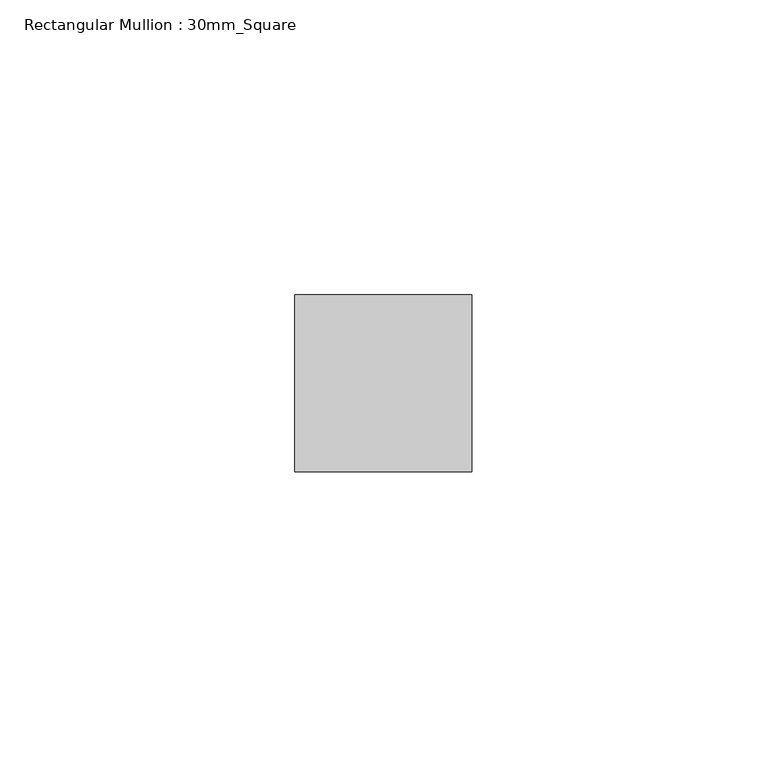
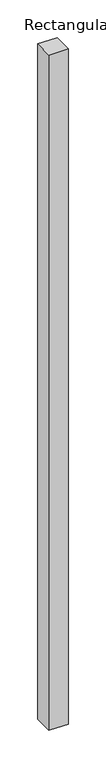
"""IFC4 building model written with IfcOpenShell, lengths in millimetres: member geometry, Rectangular Mullion : 30mm_Square."""

from ifc_helpers import new_model, si_unit, frame, origin, place, context, project, spatial, polyline, outline, extrude, source, transform, mapped, element, save


def rectangular_mullion_30mm_square_e2360202(model_context):
    return source(origin(), model_context, "Body", "SweptSolid", [
        extrude(outline(polyline([(0.0, 15.0), (0.0, -15.0), (-30.0, -15.0), (-30.0, 15.0), (0.0, 15.0)])), frame((0.0, 0.0, -1098.5425256), z_axis=(0.0, 0.0, 1.0), x_axis=(1.0, 0.0, 0.0)), (0.0, 0.0, 1.0), 1098.5425256),
    ])


if __name__ == "__main__":
    model = new_model("IFC4")
    model_context = context("Model", 3, world=origin())
    ifc_project = project(units=[si_unit("LENGTHUNIT", "METRE", prefix="MILLI")], contexts=[model_context])
    site = spatial("IfcSite", under=ifc_project)
    building = spatial("IfcBuilding", under=site)
    placement = place(None, origin())
    rectangular_mullion_30mm_square_shape = rectangular_mullion_30mm_square_e2360202(model_context)
    element("IfcMember", 1, ObjectType="Rectangular Mullion : 30mm_Square", at=placement, inside=building, context=model_context, shape_type="MappedRepresentation", body=[
        mapped(rectangular_mullion_30mm_square_shape, transform((0.0, 0.0, 0.0), x_axis=(1.0, 0.0, 0.0), y_axis=(0.0, 1.0, 0.0), z_axis=(0.0, 0.0, 1.0))),
    ])
    save(model, "model.ifc")

# Revit data of these elements
# Type "Rectangular Mullion : 30mm_Square"
#   Keynote = "H11"
#   built-in parameter 1007304 = 0.0984252 (stored number, unit not read)
#   built-in parameter 1007301 = 0.0492126 (stored number, unit not read)
#   built-in parameter 1007300 = 0.0492126 (stored number, unit not read)
# Element 1 (IfcMember, "Rectangular Mullion : 30mm_Square")
#   Materials on its faces: "Aluminium"
# Materials
#   "Aluminium": class "Metal", colour RGB 247 247 247, transparency 0, Description = "Aluminium 6061", Cost = 0
